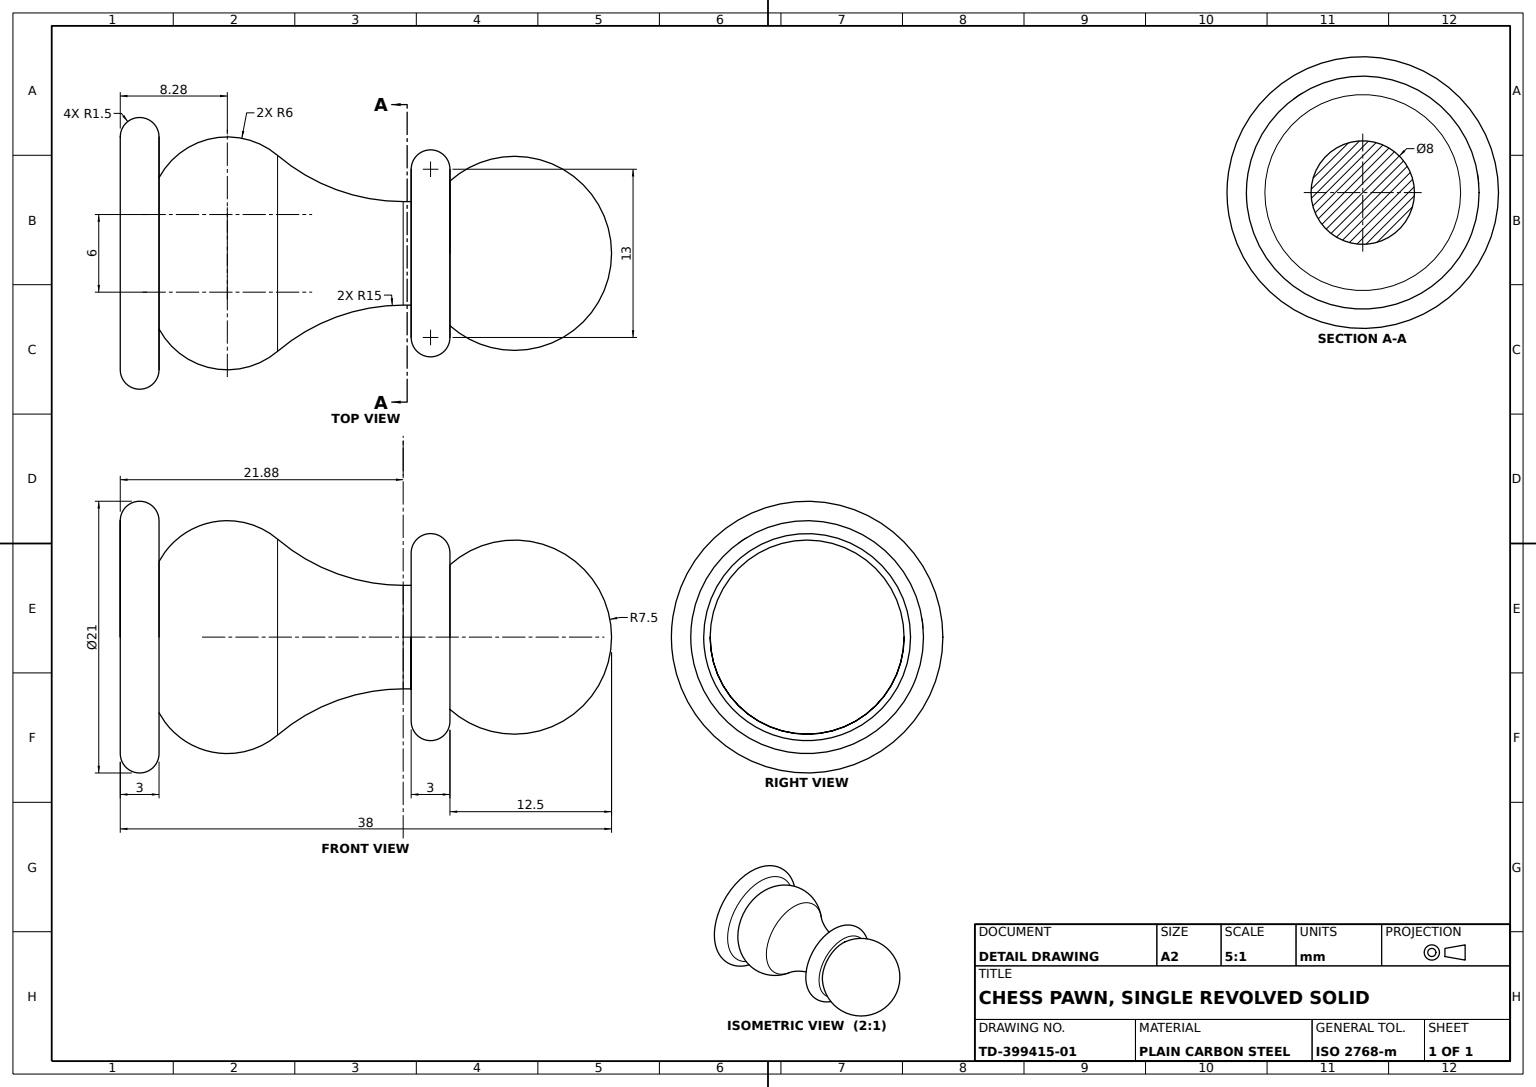
SolidWorks part; units mm, degrees
material "Plain Carbon Steel"
ref_plane "Front Plane" through (0, 0, 0) normal (0, 0, 1) x (1, 0, 0)
ref_plane "Top Plane" through (0, 0, 0) normal (0, 1, 0) x (1, 0, 0)
ref_plane "Right Plane" through (0, 0, 0) normal (1, 0, 0) x (0, 0, -1)
sketch "Pawn Profile Sketch" plane through (0, 0, 0) normal (0, 0, 1) x (1, 0, 0)
  line L0 (0, 0) -> (0, -43.7256) construction
  line L3 (0, -12.5) -> (-6.5, -12.5)
  line L5 (0, -38) -> (-9, -38)
  line L7 (-4, -15.5) -> (-4, -16.1175)
  line L12 (0, -15.5) -> (-6.5, -15.5)
  line L13 (0, -35) -> (-9, -35)
  arc A2 (-6.5, -12.5) -> (-6.5, -15.5) centre (-6.5, -14) ccw
  arc A5 (-9, -35) -> (-9, -38) centre (-9, -36.5) ccw
  arc A9 (-7.5714, -25.8329) -> (-5.848, -35) centre (-3, -29.719) ccw
  arc A10 (-4, -16.1175) -> (-7.5714, -25.8329) centre (-19, -16.1175) cw
  arc A11 (0, 0) -> (-5.5902, -12.5) centre (0, -7.5) ccw
  arc A12 (-0.152, -35) -> (0, -34.9151) centre (-3, -29.719) ccw
  point P7 (0, -14)
  point P16 (0, -36.5)
  dimension "D1" = 1.5
  dimension "D3" = 6
  dimension "D4" = 15
  dimension "D6" = 7.5
  dimension "D11" = 9
  dimension "D2" = 12.5
  dimension "D5" = 38
  dimension "D7" = 0.152
  dimension "D8" = 3
  dimension "D9" = 4
  dimension "D10" = 6.5
revolve "Pawn Body Revolve" add sketch "Pawn Profile Sketch" angle 360 about L0
